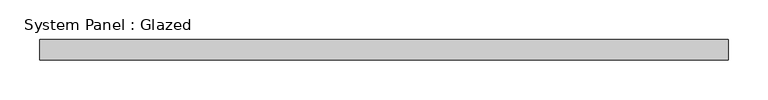
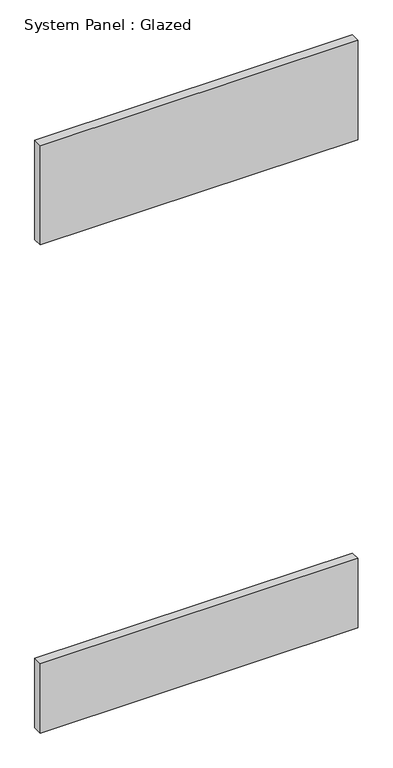
"""IFC4 building model written with IfcOpenShell, lengths in millimetres: plate geometry, System Panel : Glazed."""

from ifc_helpers import new_model, si_unit, frame, origin, origin_with_axes, place, context, project, spatial, polyline, outline, extrude, source, transform, mapped, element, save


def system_panel_glazed_a01a9dc6(model_context):
    return source(origin(), model_context, "Body", "SweptSolid", [
        extrude(outline(polyline([(432.3220098, 19.05), (-432.3220098, 19.05), (-432.3220098, 44.45), (432.3220098, 44.45), (432.3220098, 19.05)])), frame((0.0, 0.0, 1403.35), z_axis=(0.0, 0.0, 1.0), x_axis=(1.0, 0.0, 0.0)), (0.0, 0.0, 1.0), 285.75),
        extrude(outline(polyline([(432.3220098, 19.05), (-432.3220098, 19.05), (-432.3220098, 44.45), (432.3220098, 44.45), (432.3220098, 19.05)])), origin_with_axes(), (0.0, 0.0, 1.0), 199.39),
    ])


if __name__ == "__main__":
    model = new_model("IFC4")
    model_context = context("Model", 3, world=origin())
    ifc_project = project(units=[si_unit("LENGTHUNIT", "METRE", prefix="MILLI")], contexts=[model_context])
    site = spatial("IfcSite", under=ifc_project)
    building = spatial("IfcBuilding", under=site)
    placement = place(None, origin())
    system_panel_glazed_shape = system_panel_glazed_a01a9dc6(model_context)
    element("IfcPlate", 1, ObjectType="System Panel : Glazed", at=placement, inside=building, context=model_context, shape_type="MappedRepresentation", body=[
        mapped(system_panel_glazed_shape, transform((0.0, 0.0, 0.0), x_axis=(1.0, 0.0, 0.0), y_axis=(0.0, 1.0, 0.0), z_axis=(0.0, 0.0, 1.0))),
    ])
    save(model, "model.ifc")

# Revit data of these elements
# Type "System Panel : Glazed"
#   Construction Type Id = "GSP4R"
#   Analytic Construction = "1/8 in Pilkington single glazing"
#   Visual Light Transmittance = 0.9
#   Solar Heat Gain Coefficient = 0.86
#   Heat Transfer Coefficient (U) = 1.18115 BTU/(h·ft²·°F)
#   Define Thermal Properties by = 1
# Element 1 (IfcPlate, "System Panel : Glazed")
#   Materials on its faces: "Glass"
# Materials
#   "Glass": class "Glass", colour RGB 0 128 192, transparency 0.75, Description = "Soda Lime Glass", Cost = 0
